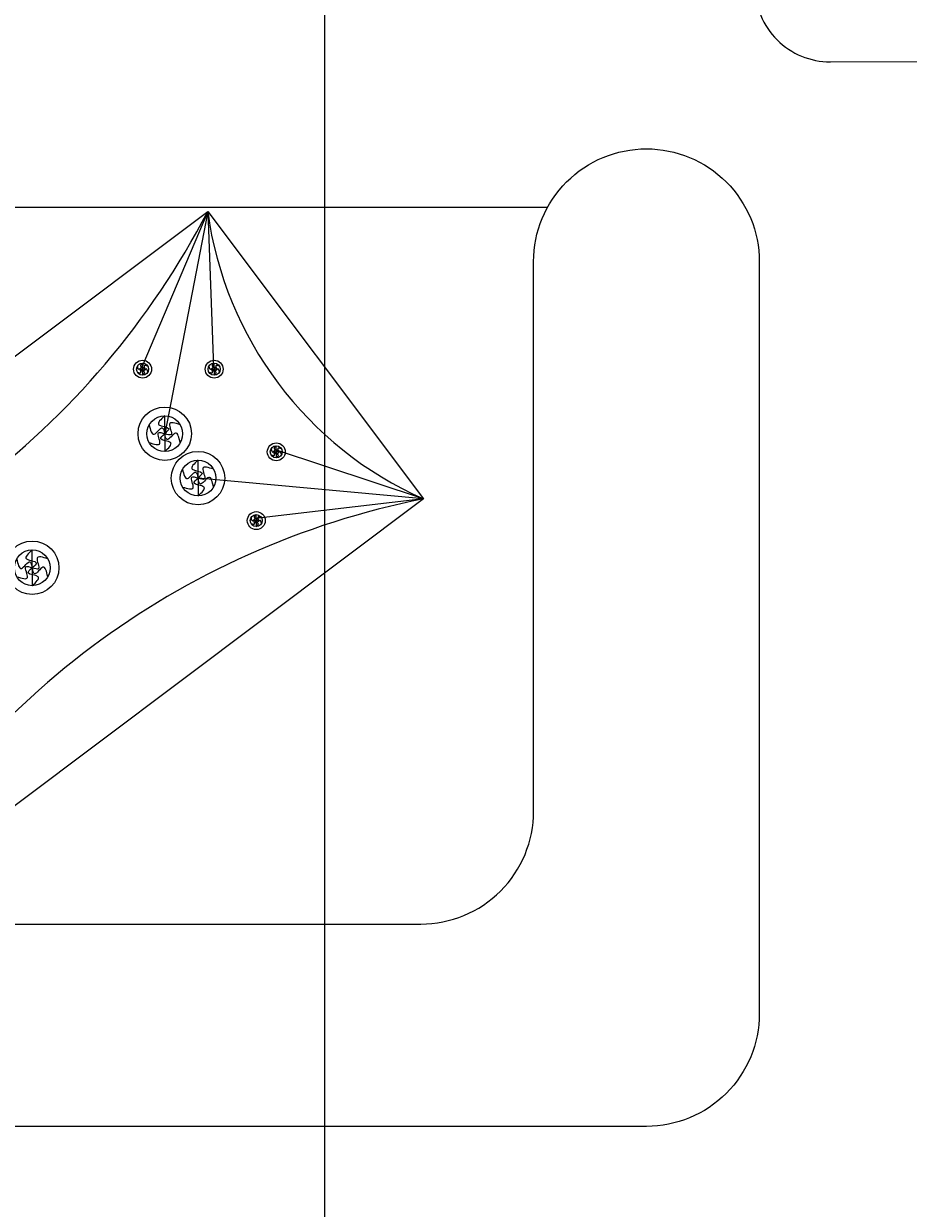
# Model space of a CAD drawing. Units: inches. Extents: x -61 to 1599, y -1316 to 257.
# Tile 134 of 204: x 484 to 507, y -166 to -135. Entities that reach past the tile are written whole.
import ezdxf

# ---------------------------------------------------------------- set-up
doc = ezdxf.new("R2010")
doc.units = ezdxf.units.IN
doc.header["$MEASUREMENT"] = 0
doc.layers.add('A-ANNO-DIMS', color=2, linetype='Continuous', lineweight=18)
doc.layers.add('FURNITURE', color=83, linetype='Continuous', lineweight=18)
doc.layers.add('FUR', color=83, linetype='Continuous')
doc.styles.get("Standard").update_dxf_attribs({"font": 'arial.ttf'})
doc.dimstyles.get("Standard").update_dxf_attribs({"dimtxt": 0.18, "dimasz": 0.18, "dimexe": 0.18, "dimexo": 0.0625, "dimgap": 0.09, "dimtad": 0, "dimtih": 1, "dimtoh": 1, "dimdec": 0, "dimzin": 0, "dimdsep": 46, "dimlunit": 3, "dimtxsty": 'Standard', "dimcen": 0.09, "dimadec": 0, "dimazin": 0, "dimtfac": 1, "dimtdec": 0, "dimtofl": 0, "dimtmove": 0, "dimatfit": 3, "dimfxl": 1, "dimtolj": 1, "dimtzin": 0, "dimarcsym": 0})

# ---------------------------------------------------------------- blocks, each defined once
blk = doc.blocks.new('*U156')
at = {"layer": 'FUR'}
blk.add_open_spline([(0.015, 0.238), (-0.088, 0.143), (-0.292, -0.045), (0.224, -0.053), (0.072, -0.187), (0.015, -0.238)], degree=3, knots=[0, 0, 0, 0, 0.2846533, 0.5662105, 0.736751, 0.736751, 0.736751, 0.736751], dxfattribs=at)
blk = doc.blocks.new('*U157')
at = {"layer": 'FUR', "transparency": 16777216}
blk.add_blockref('*U156', (662.716, -238.357), dxfattribs=at)
for p, rotation in [((662.929, -238.463), 300), ((662.517, -238.489), 60), ((662.531, -238.727), 120), ((662.944, -238.702), 240), ((662.745, -238.833), 180)]:
    blk.add_blockref('*U156', p, dxfattribs=dict(at, rotation=rotation))
blk = doc.blocks.new('*U120')
at = {"layer": 'FUR'}
blk.add_open_spline([(0.005, 0.08), (-0.03, 0.048), (-0.098, -0.015), (0.075, -0.018), (0.024, -0.063), (0.005, -0.08)], degree=3, knots=[0, 0, 0, 0, 0.0954578, 0.1898773, 0.2470677, 0.2470677, 0.2470677, 0.2470677], dxfattribs=at)
blk = doc.blocks.new('*U121')
at = {"layer": 'FUR', "transparency": 16777216}
for p, rotation in [((222.173, -79.977), 60), ((222.178, -80.056), 120), ((222.25, -80.092), 180), ((222.312, -79.968), 300), ((222.317, -80.048), 240)]:
    blk.add_blockref('*U120', p, dxfattribs=dict(at, rotation=rotation))
blk.add_blockref('*U120', (222.24, -79.932), dxfattribs=at)
blk = doc.blocks.new('*U140')
at = {"layer": 'FUR'}
blk.add_open_spline([(0.015, 0.238), (-0.088, 0.143), (-0.292, -0.045), (0.224, -0.053), (0.072, -0.187), (0.015, -0.238)], degree=3, knots=[0, 0, 0, 0, 0.2846533, 0.5662105, 0.736751, 0.736751, 0.736751, 0.736751], dxfattribs=at)
blk = doc.blocks.new('*U141')
at = {"layer": 'FUR', "transparency": 16777216}
blk.add_blockref('*U140', (662.716, -238.357), dxfattribs=at)
for p, rotation in [((662.929, -238.463), 300), ((662.517, -238.489), 60), ((662.531, -238.727), 120), ((662.944, -238.702), 240), ((662.745, -238.833), 180)]:
    blk.add_blockref('*U140', p, dxfattribs=dict(at, rotation=rotation))
blk = doc.blocks.new('*U135')
at = {"layer": 'FUR'}
blk.add_open_spline([(0.015, 0.238), (-0.088, 0.143), (-0.292, -0.045), (0.224, -0.053), (0.072, -0.187), (0.015, -0.238)], degree=3, knots=[0, 0, 0, 0, 0.2846533, 0.5662105, 0.736751, 0.736751, 0.736751, 0.736751], dxfattribs=at)
blk = doc.blocks.new('*U136')
at = {"layer": 'FUR', "transparency": 16777216}
blk.add_blockref('*U135', (662.716, -238.357), dxfattribs=at)
for p, rotation in [((662.929, -238.463), 300), ((662.517, -238.489), 60), ((662.531, -238.727), 120), ((662.944, -238.702), 240), ((662.745, -238.833), 180)]:
    blk.add_blockref('*U135', p, dxfattribs=dict(at, rotation=rotation))
blk = doc.blocks.new('*U118')
at = {"layer": 'FUR'}
blk.add_open_spline([(0.005, 0.08), (-0.03, 0.048), (-0.098, -0.015), (0.075, -0.018), (0.024, -0.063), (0.005, -0.08)], degree=3, knots=[0, 0, 0, 0, 0.0954578, 0.1898773, 0.2470677, 0.2470677, 0.2470677, 0.2470677], dxfattribs=at)
blk = doc.blocks.new('*U119')
at = {"layer": 'FUR', "transparency": 16777216}
for p, rotation in [((222.173, -79.977), 60), ((222.178, -80.056), 120), ((222.25, -80.092), 180), ((222.312, -79.968), 300), ((222.317, -80.048), 240)]:
    blk.add_blockref('*U118', p, dxfattribs=dict(at, rotation=rotation))
blk.add_blockref('*U118', (222.24, -79.932), dxfattribs=at)
blk = doc.blocks.new('*U138')
at = {"layer": 'FUR'}
blk.add_open_spline([(0.005, 0.08), (-0.03, 0.048), (-0.098, -0.015), (0.075, -0.018), (0.024, -0.063), (0.005, -0.08)], degree=3, knots=[0, 0, 0, 0, 0.0954578, 0.1898773, 0.2470677, 0.2470677, 0.2470677, 0.2470677], dxfattribs=at)
blk = doc.blocks.new('*U139')
at = {"layer": 'FUR', "transparency": 16777216}
for p, rotation in [((222.173, -79.977), 60), ((222.178, -80.056), 120), ((222.25, -80.092), 180), ((222.312, -79.968), 300), ((222.317, -80.048), 240)]:
    blk.add_blockref('*U138', p, dxfattribs=dict(at, rotation=rotation))
blk.add_blockref('*U138', (222.24, -79.932), dxfattribs=at)
blk = doc.blocks.new('*U122')
at = {"layer": 'FUR'}
blk.add_open_spline([(0.005, 0.08), (-0.03, 0.048), (-0.098, -0.015), (0.075, -0.018), (0.024, -0.063), (0.005, -0.08)], degree=3, knots=[0, 0, 0, 0, 0.0954578, 0.1898773, 0.2470677, 0.2470677, 0.2470677, 0.2470677], dxfattribs=at)
blk = doc.blocks.new('*U137')
at = {"layer": 'FUR', "transparency": 16777216}
for p, rotation in [((222.173, -79.977), 60), ((222.178, -80.056), 120), ((222.25, -80.092), 180), ((222.312, -79.968), 300), ((222.317, -80.048), 240)]:
    blk.add_blockref('*U122', p, dxfattribs=dict(at, rotation=rotation))
blk.add_blockref('*U122', (222.24, -79.932), dxfattribs=at)
blk = doc.blocks.new('SOFA-THREE-SEAT')
for p, q in [((78.369, 24.442), (57, 24.442)), ((69.336, 24.333), (67.586, 20.192)), ((69.336, 24.333), (68.194, 18.423)), ((69.336, 24.333), (69.49, 20.192)), ((67.605, 20.139), (67.605, 20.299)), ((69.509, 20.139), (69.509, 20.299)), ((67.605, 20.139), (67.605, 19.979)), ((69.509, 20.139), (69.509, 19.979)), ((68.194, 18.423), (68.194, 18.899)), ((68.194, 18.423), (68.194, 17.946)), ((75.074, 16.687), (71.14, 17.993)), ((71.159, 17.94), (71.159, 18.1)), ((69.079, 17.243), (69.079, 17.719)), ((71.159, 17.94), (71.159, 17.78)), ((75.074, 16.687), (69.079, 17.243)), ((69.079, 17.243), (69.079, 16.766)), ((75.074, 16.687), (70.608, 16.164)), ((70.627, 16.112), (70.627, 16.272)), ((70.627, 16.112), (70.627, 15.952)), ((64.672, 14.857), (64.672, 15.334)), ((64.672, 14.857), (64.672, 14.381))]:
    blk.add_line(p, q)
blk.add_lwpolyline([(78, 8.382), (78, 23, -0.414214), (81, 26), (81, 26, -0.414214), (84, 23), (84, 3, -0.414214), (81, 0), (3, 0, -0.414214), (0, 3), (0, 23, -0.414214), (3, 26), (3, 26, -0.414214), (6, 23), (6, 8.382, 0.414214), (9, 5.382), (75, 5.382, 0.414214)], format="xyb", close=True)
blk.add_lwpolyline([(54.271, 13.028), (69.336, 24.333), (75.074, 16.687), (60.009, 5.382)], close=True)
for centre, radius in [((67.605, 20.139), 0.238), ((67.605, 20.139), 0.16), ((69.509, 20.139), 0.238), ((69.509, 20.139), 0.16), ((68.194, 18.423), 0.71), ((68.194, 18.423), 0.476), ((71.159, 17.94), 0.238), ((71.159, 17.94), 0.16), ((69.079, 17.243), 0.71), ((69.079, 17.243), 0.476), ((70.627, 16.112), 0.238), ((70.627, 16.112), 0.16), ((64.672, 14.857), 0.71), ((64.672, 14.857), 0.476)]:
    blk.add_circle(centre, radius)
for centre, radius, start, end in [((50.048, 34.345), 21.731, 281.2044, 332.5684), ((79.062, 25.656), 9.816, 187.747, 246.0258), ((79.296, -4.63), 21.731, 101.2044, 152.5684)]:
    blk.add_arc(centre, radius, start, end)
at = {"rotation": 180}
for name, p in [('*U121', (289.85, -59.873)), ('*U119', (291.754, -59.873)), ('*U141', (730.924, -220.172)), ('*U137', (293.404, -62.072)), ('*U136', (731.81, -221.352)), ('*U139', (292.872, -63.9)), ('*U157', (727.402, -223.738))]:
    blk.add_blockref(name, p, dxfattribs=at)
blk = doc.blocks.new('*D704')
at = {"layer": 'A-ANNO-DIMS', "color": 0, "lineweight": -2, "transparency": 16777216}
for p, q in [((491.833, -616.882), (491.833, 257.457)), ((544.703, -616.882), (544.703, 257.457)), ((492.013, 257.277), (517.874, 257.277)), ((544.523, 257.277), (518.661, 257.277))]:
    blk.add_line(p, q, dxfattribs=at)
at = {"layer": 'A-ANNO-DIMS', "color": 0, "transparency": 16777216}
for points in [[(492.013, 257.307), (492.013, 257.247), (491.833, 257.277)], [(544.523, 257.307), (544.523, 257.247), (544.703, 257.277)]]:
    blk.add_solid(points, dxfattribs=at)
at = {"layer": 'DEFPOINTS', "color": 0, "transparency": 16777216}
for p in [(544.703, 257.277), (491.833, -616.945), (544.703, -616.945)]:
    blk.add_point(p, dxfattribs=at)
at = {"layer": 'A-ANNO-DIMS', "color": 0, "transparency": 16777216, "insert": (518.268, 257.277), "char_height": 0.18, "attachment_point": 5}
blk.add_mtext('\\A1;52.87', dxfattribs=at)

msp = doc.modelspace()

# ---------------------------------------------------------------- linework, layer by layer
at = {"layer": 'FURNITURE'}
msp.add_lwpolyline([(503.2659, -129.8197), (503.2714, -133.8197, 0.4142136), (505.2742, -135.817), (527.2741, -135.7867, 0.4142137), (529.2714, -133.784), (529.1944, -77.784, 0.4142134), (527.1916, -75.7868), (505.1917, -75.817, 0.4142136), (503.1944, -77.8197), (503.1999, -81.8197)], format="xyb", dxfattribs=at)

# ---------------------------------------------------------------- block references
msp.add_blockref('SOFA-THREE-SEAT', (419.3851, -164.1303), dxfattribs=at)

# ---------------------------------------------------------------- dimensions: what is measured, and where the dimension line sits
at = {"layer": 'A-ANNO-DIMS'}
dim = msp.add_linear_dim(base=(544.7028, 257.2771), p1=(491.8327, -616.9446), p2=(544.7028, -616.9446), dimstyle='Standard', override={"dimdec": 2, "dimlfac": 1, "dimrnd": 0, "dimzin": 0, "dimdsep": 46, "dimlunit": 2}, dxfattribs=at)
dim.commit()
dim.dimension.update_dxf_attribs({"geometry": '*D704', "text_midpoint": (518.2677, 257.2771)})

doc.saveas('drawing.dxf')
